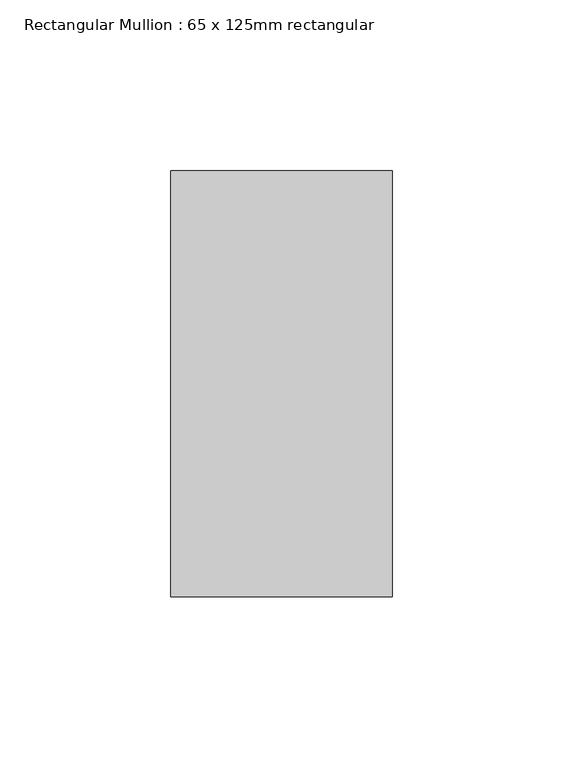
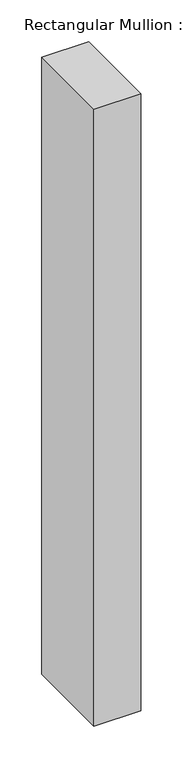
"""IFC4 building model written with IfcOpenShell, lengths in millimetres: member geometry, Rectangular Mullion : 65 x 125mm rectangular."""

from ifc_helpers import new_model, si_unit, frame, origin, place, context, project, spatial, polyline, outline, extrude, source, transform, mapped, element, save


def rectangular_mullion_65_x_125mm_rectangular_018360c9(model_context):
    return source(origin(), model_context, "Body", "SweptSolid", [
        extrude(outline(polyline([(32.5, 62.5), (32.5, -62.5), (-32.5, -62.5), (-32.5, 62.5), (32.5, 62.5)])), frame((0.0, 0.0, -902.5), z_axis=(0.0, 0.0, 1.0), x_axis=(1.0, 0.0, 0.0)), (0.0, 0.0, 1.0), 902.5),
    ])


if __name__ == "__main__":
    model = new_model("IFC4")
    model_context = context("Model", 3, world=origin())
    ifc_project = project(units=[si_unit("LENGTHUNIT", "METRE", prefix="MILLI")], contexts=[model_context])
    site = spatial("IfcSite", under=ifc_project)
    building = spatial("IfcBuilding", under=site)
    placement = place(None, origin())
    rectangular_mullion_65_x_125mm_rectangular_shape = rectangular_mullion_65_x_125mm_rectangular_018360c9(model_context)
    element("IfcMember", 1, ObjectType="Rectangular Mullion : 65 x 125mm rectangular", at=placement, inside=building, context=model_context, shape_type="MappedRepresentation", body=[
        mapped(rectangular_mullion_65_x_125mm_rectangular_shape, transform((0.0, 0.0, 0.0), x_axis=(1.0, 0.0, 0.0), y_axis=(0.0, 1.0, 0.0), z_axis=(0.0, 0.0, 1.0))),
    ])
    save(model, "model.ifc")

# Revit data of these elements
# Type "Rectangular Mullion : 65 x 125mm rectangular"
#   built-in parameter 1007304 = 0.410105 (stored number, unit not read)
#   built-in parameter 1007301 = 0.106627 (stored number, unit not read)
#   built-in parameter 1007300 = 0.106627 (stored number, unit not read)
# Element 1 (IfcMember, "Rectangular Mullion : 65 x 125mm rectangular")
#   Materials on its faces: "Aluminum"
# Materials
#   "Aluminum": class "Metal", colour RGB 244 245 246, transparency 0, Description = "Aluminum 6061", Cost = 0
